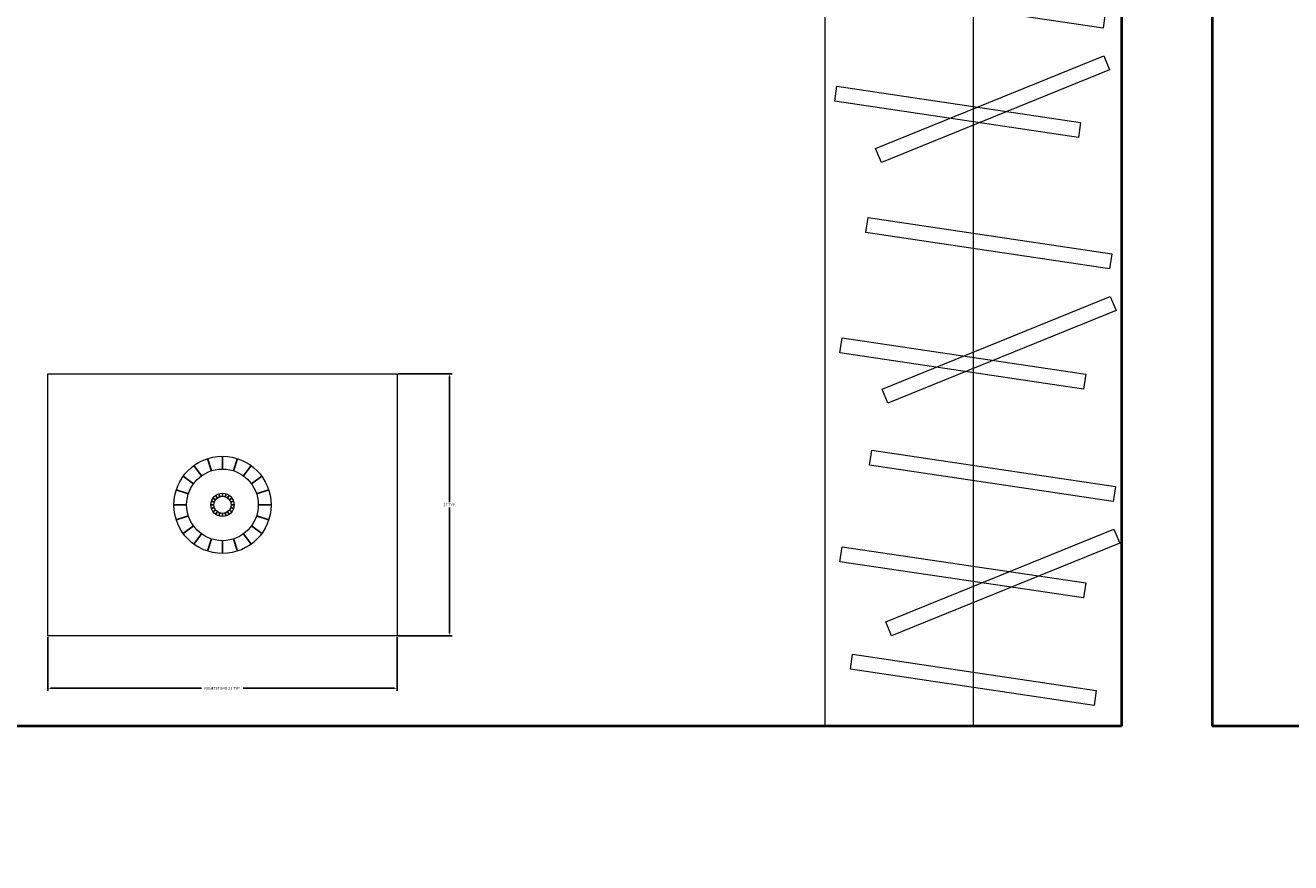
# Model space of a CAD drawing. Units: inches. Extents: x -46 to 1145, y -527 to 760.
# Tile 31 of 57: x 111 to 195, y 222 to 277. Entities that reach past the tile are written whole.
import ezdxf

# ---------------------------------------------------------------- set-up
doc = ezdxf.new("R2010")
doc.units = ezdxf.units.IN
doc.header["$MEASUREMENT"] = 0
for name, color, linetype, lineweight in [('A-ANNO-DIMS', 2, 'Continuous', 18), ('A-FLOR-CASE', 32, 'Continuous', 18), ('A-FURN', 2, 'Continuous', 13), ('WALLS', 4, 'Continuous', 40)]:
    doc.layers.add(name, color=color, linetype=linetype, lineweight=lineweight)
doc.layers.add('FURNTIURE', color=2, linetype='Continuous')
doc.styles.get("Standard").update_dxf_attribs({"font": 'arial.ttf'})
doc.dimstyles.get("Standard").update_dxf_attribs({"dimtxt": 0.18, "dimasz": 0.18, "dimexe": 0.18, "dimexo": 0.0625, "dimgap": 0.09, "dimtad": 0, "dimtih": 1, "dimtoh": 1, "dimdec": 0, "dimzin": 0, "dimdsep": 46, "dimlunit": 3, "dimtxsty": 'Standard', "dimcen": 0.09, "dimadec": 0, "dimazin": 0, "dimtfac": 1, "dimtdec": 0, "dimtofl": 0, "dimtmove": 0, "dimatfit": 3, "dimfxl": 1, "dimtolj": 1, "dimtzin": 0, "dimarcsym": 0})

# ---------------------------------------------------------------- blocks, each defined once
blk = doc.blocks.new('*U89')
at = {"layer": 'FURNTIURE'}
blk.add_line((0, 0.422), (0, -0.422), dxfattribs=at)
blk = doc.blocks.new('*U90')
at = {"layer": 'FURNTIURE', "transparency": 16777216}
for p, rotation in [((590.891, 507.397), 17.99999999999997), ((592.613, 507.397), 341.9999999999999), ((590.114, 507.002), 36), ((593.39, 507.002), 324), ((589.498, 506.385), 54), ((594.007, 506.385), 306), ((589.102, 505.608), 72), ((594.402, 505.608), 288), ((588.965, 504.747), 90), ((594.539, 504.747), 270), ((589.102, 503.886), 108), ((594.402, 503.886), 252), ((589.498, 503.109), 126), ((590.114, 502.493), 144), ((593.39, 502.493), 216), ((594.007, 503.109), 234), ((590.891, 502.097), 162), ((591.752, 501.961), 180), ((592.613, 502.097), 197.9999999999999)]:
    blk.add_blockref('*U89', p, dxfattribs=dict(at, rotation=rotation))
blk.add_blockref('*U89', (591.752, 507.534), dxfattribs=at)
blk = doc.blocks.new('*U87')
at = {"layer": 'FURNTIURE'}
blk.add_line((0, 0.101), (0, -0.101), dxfattribs=at)
blk = doc.blocks.new('*U88')
at = {"layer": 'FURNTIURE', "transparency": 16777216}
for p, rotation in [((141.267, 121.245), 72), ((141.362, 121.431), 54), ((141.51, 121.579), 35.99999999999999), ((141.696, 121.674), 17.99999999999998), ((142.109, 121.674), 342), ((142.295, 121.579), 324), ((142.443, 121.431), 306), ((142.538, 121.245), 288), ((141.234, 121.039), 90), ((141.267, 120.832), 108), ((141.362, 120.646), 126), ((141.51, 120.498), 144), ((141.696, 120.403), 162), ((141.902, 120.37), 180), ((142.109, 120.403), 198), ((142.295, 120.498), 216), ((142.443, 120.646), 234), ((142.538, 120.832), 252), ((142.571, 121.039), 270)]:
    blk.add_blockref('*U87', p, dxfattribs=dict(at, rotation=rotation))
blk.add_blockref('*U87', (141.902, 121.707), dxfattribs=at)
blk = doc.blocks.new('NIGHTSTAND')
blk.add_lwpolyline([(23.061, 0), (0, 0), (0, 17.285), (23.061, 17.285)], close=True)
for radius in [3.209, 2.364, 0.77, 0.567]:
    blk.add_circle((11.53, 8.643), radius)
for name, p in [('*U90', (-580.222, -496.105)), ('*U88', (-130.372, -112.396))]:
    blk.add_blockref(name, p)
blk = doc.blocks.new('WARDROBE')
blk.add_line((9.78, 0), (9.78, 83.246))
for points in [[(19.56, 0), (0, 0), (0, 83.246), (19.56, 83.246)], [(17.735, 78.486), (1.657, 80.876), (1.804, 81.869), (17.883, 79.479)], [(15.55, 76.351), (0.491, 70.229), (0.113, 71.159), (15.172, 77.281)], [(18.434, 71.396), (2.355, 73.786), (2.502, 74.779), (18.581, 72.389)], [(16.473, 65.03), (0.395, 67.42), (0.542, 68.413), (16.621, 66.023)], [(15.79, 61.003), (0.731, 54.88), (0.353, 55.81), (15.411, 61.933)], [(18.434, 57.618), (2.355, 60.008), (2.502, 61.001), (18.581, 58.611)], [(16.713, 49.682), (0.634, 52.071), (0.782, 53.064), (16.861, 50.674)], [(16.218, 45.124), (1.16, 39.002), (0.782, 39.931), (15.84, 46.054)], [(18.771, 41.016), (2.692, 43.406), (2.839, 44.399), (18.918, 42.009)], [(17.142, 33.803), (1.063, 36.193), (1.211, 37.186), (17.29, 34.796)], [(16.647, 30.67), (1.589, 24.548), (1.211, 25.477), (16.269, 31.6)], [(17.519, 26.78), (1.441, 29.169), (1.588, 30.162), (17.667, 27.772)], [(17.571, 19.349), (1.492, 21.739), (1.64, 22.732), (17.718, 20.342)], [(17.076, 15.353), (2.018, 9.231), (1.64, 10.161), (16.698, 16.283)], [(18, 4.032), (1.921, 6.422), (2.068, 7.415), (18.147, 5.025)], [(18.324, 0.979), (2.068, 0.979), (2.068, 1.983), (18.324, 1.983)]]:
    blk.add_lwpolyline(points, close=True)
blk = doc.blocks.new('*D654')
at = {"layer": 'A-ANNO-DIMS', "color": 0, "lineweight": -2, "transparency": 16777216}
for p, q in [((112.711, 236.422), (112.711, 232.846)), ((135.771, 236.422), (135.771, 232.846)), ((112.891, 233.026), (122.865, 233.026)), ((135.591, 233.026), (125.617, 233.026))]:
    blk.add_line(p, q, dxfattribs=at)
at = {"layer": 'A-ANNO-DIMS', "color": 0, "transparency": 16777216}
for points in [[(112.891, 233.056), (112.891, 232.996), (112.711, 233.026)], [(135.591, 233.056), (135.591, 232.996), (135.771, 233.026)]]:
    blk.add_solid(points, dxfattribs=at)
at = {"layer": 'Defpoints', "color": 0, "transparency": 16777216}
for p in [(112.711, 236.485), (135.771, 236.485), (112.711, 233.026)]:
    blk.add_point(p, dxfattribs=at)
at = {"layer": 'A-ANNO-DIMS', "color": 0, "transparency": 16777216, "insert": (124.241, 233.026), "char_height": 0.18, "attachment_point": 5}
blk.add_mtext('\\A1;NIGHTSTAND 23 TYP.', dxfattribs=at)
blk = doc.blocks.new('*D655')
at = {"layer": 'A-ANNO-DIMS', "color": 0, "lineweight": -2, "transparency": 16777216}
for p, q in [((135.834, 253.77), (139.41, 253.77)), ((139.23, 253.59), (139.23, 245.308)), ((139.23, 236.665), (139.23, 244.947)), ((135.834, 236.485), (139.41, 236.485))]:
    blk.add_line(p, q, dxfattribs=at)
at = {"layer": 'A-ANNO-DIMS', "color": 0, "transparency": 16777216}
for points in [[(139.2, 253.59), (139.26, 253.59), (139.23, 253.77)], [(139.2, 236.665), (139.26, 236.665), (139.23, 236.485)]]:
    blk.add_solid(points, dxfattribs=at)
at = {"layer": 'Defpoints', "color": 0, "transparency": 16777216}
for p in [(135.771, 253.77), (135.771, 236.485), (139.23, 236.485)]:
    blk.add_point(p, dxfattribs=at)
at = {"layer": 'A-ANNO-DIMS', "color": 0, "transparency": 16777216, "insert": (139.23, 245.127), "char_height": 0.18, "attachment_point": 5}
blk.add_mtext('\\A1;17 TYP.', dxfattribs=at)
blk = doc.blocks.new('*D685')
at = {"layer": 'A-ANNO-DIMS', "color": 0, "lineweight": -2, "transparency": 16777216}
for p, q in [((183.501, 700.889), (-46.216, 700.889)), ((-46.036, 700.709), (-46.036, 116.385)), ((-46.036, -468.302), (-46.036, 116.021)), ((12.501, -468.482), (-46.216, -468.482))]:
    blk.add_line(p, q, dxfattribs=at)
at = {"layer": 'A-ANNO-DIMS', "color": 0, "transparency": 16777216}
for points in [[(-46.066, 700.709), (-46.006, 700.709), (-46.036, 700.889)], [(-46.066, -468.302), (-46.006, -468.302), (-46.036, -468.482)]]:
    blk.add_solid(points, dxfattribs=at)
at = {"layer": 'Defpoints', "color": 0, "transparency": 16777216}
for p in [(-46.036, 700.889), (183.564, 700.889), (12.564, -468.482)]:
    blk.add_point(p, dxfattribs=at)
at = {"layer": 'A-ANNO-DIMS', "color": 0, "transparency": 16777216, "insert": (-46.036, 116.203), "char_height": 0.18, "attachment_point": 5}
blk.add_mtext('\\A1;1169.4', dxfattribs=at)

msp = doc.modelspace()

# ---------------------------------------------------------------- linework, layer by layer
at = {"layer": 'WALLS'}
for p, q in [((183.5637, 325.5663), (183.5637, 230.5176)), ((189.5637, 325.5613), (189.5637, 230.5176)), ((183.5637, 230.5176), (21.5637, 230.5176)), ((209.8481, 230.5176), (189.5637, 230.5176))]:
    msp.add_line(p, q, dxfattribs=at)

# ---------------------------------------------------------------- block references
at = {"layer": 'A-FLOR-CASE', "rotation": 180}
msp.add_blockref('WARDROBE', (183.5642, 313.7631), dxfattribs=at)
at = {"layer": 'A-FURN', "rotation": 180}
msp.add_blockref('NIGHTSTAND', (135.7717, 253.7698), dxfattribs=at)

# ---------------------------------------------------------------- dimensions: what is measured, and where the dimension line sits
at = {"layer": 'A-ANNO-DIMS'}
dim = msp.add_linear_dim(base=(-46.0363, 700.8886), p1=(12.5637, -468.4824), p2=(183.5637, 700.8886), angle=90, dimstyle='Standard', override={"dimdec": 1, "dimlfac": 1, "dimrnd": 0, "dimzin": 0, "dimdsep": 46, "dimlunit": 2}, dxfattribs=at)
dim.commit()
dim.dimension.update_dxf_attribs({"geometry": '*D685', "text_midpoint": (-46.0363, 116.2031)})
for base, p1, p2, angle, text, picture, middle in [((139.2305, 236.4848), (135.7714, 253.7697), (135.7714, 236.4848), 270, '<> TYP.', '*D655', (139.2305, 245.1272)), ((112.7111, 233.0258), (135.7714, 236.4848), (112.7111, 236.4848), 180, 'NIGHTSTAND <> TYP.', '*D654', (124.2413, 233.0258))]:
    dim = msp.add_linear_dim(base=base, p1=p1, p2=p2, angle=angle, text=text, dimstyle='Standard', override={"dimdec": 0, "dimlfac": 1, "dimrnd": 0, "dimzin": 0, "dimdsep": 46, "dimlunit": 2}, dxfattribs=at)
    dim.commit()
    dim.dimension.update_dxf_attribs({"geometry": picture, "text_midpoint": middle})

doc.saveas('drawing.dxf')
